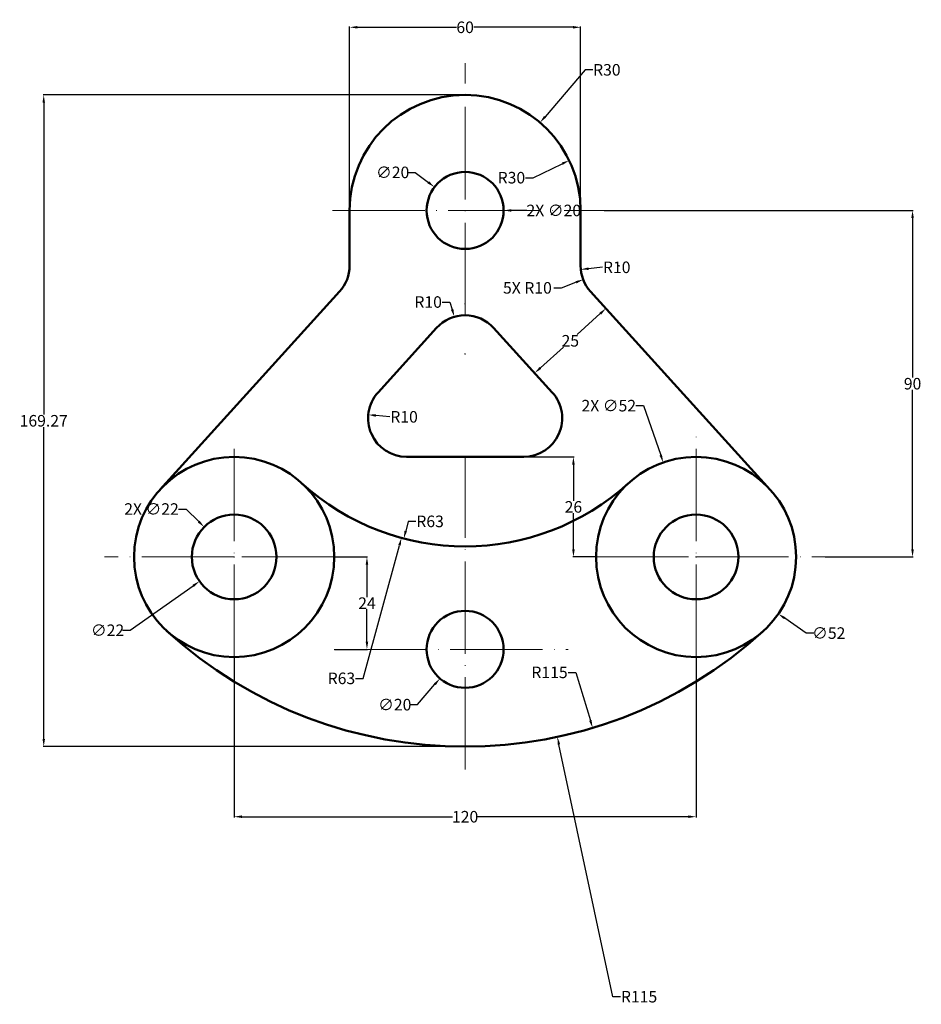
# Model space of a CAD drawing. Units: inches. Extents: x 239 to 473, y 124 to 379.
import ezdxf

# ---------------------------------------------------------------- set-up
doc = ezdxf.new("R2010")
doc.units = ezdxf.units.IN
doc.header["$MEASUREMENT"] = 0
doc.linetypes.add('ACAD_ISO04W100', pattern=[30, 24, -3, 0, -3])
for name, color, linetype, lineweight in [('M-CNTR', 4, 'ACAD_ISO04W100', 18), ('M-DIMS', 2, 'Continuous', 25), ('M-OUTL', 7, 'Continuous', 50)]:
    doc.layers.add(name, color=color, linetype=linetype, lineweight=lineweight)
doc.styles.get("Standard").update_dxf_attribs({"font": 'arial.ttf'})
doc.dimstyles.get("Standard").update_dxf_attribs({"dimtxt": 3, "dimasz": 2, "dimexe": 0.18, "dimexo": 0.0625, "dimgap": 0.09, "dimtad": 0, "dimtih": 1, "dimtoh": 1, "dimdec": 0, "dimzin": 0, "dimdsep": 46, "dimtxsty": 'Standard', "dimcen": 0.09, "dimadec": 0, "dimazin": 0, "dimtfac": 1, "dimtdec": 0, "dimtofl": 0, "dimtmove": 0, "dimatfit": 3, "dimfxl": 1, "dimtolj": 1, "dimtzin": 0, "dimarcsym": 0})

# ---------------------------------------------------------------- blocks, each defined once
blk = doc.blocks.new('*D1')
at = {"layer": 'Defpoints', "color": 0, "transparency": 16777216}
for p in [(381.57, 342.88), (354.54, 329.88)]:
    blk.add_point(p, dxfattribs=at)
at = {"layer": 'M-DIMS', "color": 0, "lineweight": -2, "transparency": 16777216}
for p, q in [((372.23, 338.39), (379.77, 342.02)), ((370.23, 338.39), (372.23, 338.39))]:
    blk.add_line(p, q, dxfattribs=at)
at = {"layer": 'M-DIMS', "color": 0, "transparency": 16777216}
blk.add_solid([(379.63, 342.32), (379.91, 341.72), (381.57, 342.88)], dxfattribs=at)
at = {"layer": 'M-DIMS', "color": 0, "transparency": 16777216, "insert": (366.56, 338.39), "char_height": 3, "attachment_point": 5}
blk.add_mtext('\\A1;R30', dxfattribs=at)
blk = doc.blocks.new('*D2')
at = {"layer": 'Defpoints', "color": 0, "transparency": 16777216}
for p in [(346.59, 335.95), (362.49, 323.82)]:
    blk.add_point(p, dxfattribs=at)
at = {"layer": 'M-DIMS', "color": 0, "lineweight": -2, "transparency": 16777216}
for p, q in [((339.58, 339.77), (341.58, 339.77)), ((341.58, 339.77), (345, 337.16)), ((354.54, 329.79), (354.54, 329.97)), ((354.45, 329.88), (354.63, 329.88))]:
    blk.add_line(p, q, dxfattribs=at)
at = {"layer": 'M-DIMS', "color": 0, "transparency": 16777216}
blk.add_solid([(345.2, 337.43), (344.79, 336.9), (346.59, 335.95)], dxfattribs=at)
at = {"layer": 'M-DIMS', "color": 0, "transparency": 16777216, "insert": (335.72, 339.77), "char_height": 3, "attachment_point": 5}
blk.add_mtext('\\A1;∅20', dxfattribs=at)
blk = doc.blocks.new('*D3')
at = {"layer": 'Defpoints', "color": 0, "transparency": 16777216}
for p in [(390.61, 329.88), (448.02, 239.88), (470.77, 239.88)]:
    blk.add_point(p, dxfattribs=at)
at = {"layer": 'M-DIMS', "color": 0, "lineweight": -2, "transparency": 16777216}
for p, q in [((390.67, 329.88), (470.95, 329.88)), ((470.77, 327.88), (470.77, 286.5)), ((470.77, 241.88), (470.77, 283.26)), ((448.08, 239.88), (470.95, 239.88))]:
    blk.add_line(p, q, dxfattribs=at)
at = {"layer": 'M-DIMS', "color": 0, "transparency": 16777216}
for points in [[(470.43, 327.88), (471.1, 327.88), (470.77, 329.88)], [(470.43, 241.88), (471.1, 241.88), (470.77, 239.88)]]:
    blk.add_solid(points, dxfattribs=at)
at = {"layer": 'M-DIMS', "color": 0, "transparency": 16777216, "insert": (470.77, 284.88), "char_height": 3, "attachment_point": 5}
blk.add_mtext('\\A1;90', dxfattribs=at)
blk = doc.blocks.new('*D4')
at = {"layer": 'Defpoints', "color": 0, "transparency": 16777216}
for p in [(354.54, 305.62), (338.61, 244.66)]:
    blk.add_point(p, dxfattribs=at)
at = {"layer": 'M-DIMS', "color": 0, "lineweight": -2, "transparency": 16777216}
for p, q in [((339.77, 249.12), (339.11, 246.6)), ((341.77, 249.12), (339.77, 249.12))]:
    blk.add_line(p, q, dxfattribs=at)
at = {"layer": 'M-DIMS', "color": 0, "transparency": 16777216}
blk.add_solid([(338.79, 246.68), (339.43, 246.52), (338.61, 244.66)], dxfattribs=at)
at = {"layer": 'M-DIMS', "color": 0, "transparency": 16777216, "insert": (345.44, 249.12), "char_height": 3, "attachment_point": 5}
blk.add_mtext('\\A1;R63', dxfattribs=at)
blk = doc.blocks.new('*D5')
at = {"layer": 'Defpoints', "color": 0, "transparency": 16777216}
for p in [(303.53, 246.22), (285.54, 233.55)]:
    blk.add_point(p, dxfattribs=at)
at = {"layer": 'M-DIMS', "color": 0, "lineweight": -2, "transparency": 16777216}
for p, q in [((294.45, 239.88), (294.63, 239.88)), ((294.54, 239.79), (294.54, 239.97)), ((267.52, 220.84), (283.91, 232.39)), ((265.52, 220.84), (267.52, 220.84))]:
    blk.add_line(p, q, dxfattribs=at)
at = {"layer": 'M-DIMS', "color": 0, "transparency": 16777216}
blk.add_solid([(283.72, 232.67), (284.1, 232.12), (285.54, 233.55)], dxfattribs=at)
at = {"layer": 'M-DIMS', "color": 0, "transparency": 16777216, "insert": (261.66, 220.84), "char_height": 3, "attachment_point": 5}
blk.add_mtext('\\A1;∅22', dxfattribs=at)
blk = doc.blocks.new('*D6')
at = {"layer": 'Defpoints', "color": 0, "transparency": 16777216}
for p in [(393.15, 254.67), (435.92, 225.1)]:
    blk.add_point(p, dxfattribs=at)
at = {"layer": 'M-DIMS', "color": 0, "lineweight": -2, "transparency": 16777216}
for p, q in [((414.45, 239.88), (414.63, 239.88)), ((414.54, 239.79), (414.54, 239.97)), ((443.13, 220.11), (437.57, 223.96)), ((445.13, 220.11), (443.13, 220.11))]:
    blk.add_line(p, q, dxfattribs=at)
at = {"layer": 'M-DIMS', "color": 0, "transparency": 16777216}
blk.add_solid([(437.76, 224.23), (437.38, 223.68), (435.92, 225.1)], dxfattribs=at)
at = {"layer": 'M-DIMS', "color": 0, "transparency": 16777216, "insert": (448.99, 220.11), "char_height": 3, "attachment_point": 5}
blk.add_mtext('\\A1;∅52', dxfattribs=at)
blk = doc.blocks.new('*D7')
at = {"layer": 'Defpoints', "color": 0, "transparency": 16777216}
for p in [(354.54, 305.62), (387.65, 195.49)]:
    blk.add_point(p, dxfattribs=at)
at = {"layer": 'M-DIMS', "color": 0, "lineweight": -2, "transparency": 16777216}
for p, q in [((381.31, 209.9), (383.31, 209.9)), ((383.31, 209.9), (387.07, 197.4))]:
    blk.add_line(p, q, dxfattribs=at)
at = {"layer": 'M-DIMS', "color": 0, "transparency": 16777216}
blk.add_solid([(387.39, 197.5), (386.75, 197.31), (387.65, 195.49)], dxfattribs=at)
at = {"layer": 'M-DIMS', "color": 0, "transparency": 16777216, "insert": (376.46, 209.9), "char_height": 3, "attachment_point": 5}
blk.add_mtext('\\A1;R115', dxfattribs=at)
blk = doc.blocks.new('*D8')
at = {"layer": 'Defpoints', "color": 0, "transparency": 16777216}
for p in [(361.07, 223.45), (348, 208.32)]:
    blk.add_point(p, dxfattribs=at)
at = {"layer": 'M-DIMS', "color": 0, "lineweight": -2, "transparency": 16777216}
for p, q in [((354.45, 215.88), (354.63, 215.88)), ((354.54, 215.79), (354.54, 215.97)), ((342.13, 201.52), (346.69, 206.8)), ((340.13, 201.52), (342.13, 201.52))]:
    blk.add_line(p, q, dxfattribs=at)
at = {"layer": 'M-DIMS', "color": 0, "transparency": 16777216}
blk.add_solid([(346.44, 207.02), (346.94, 206.58), (348, 208.32)], dxfattribs=at)
at = {"layer": 'M-DIMS', "color": 0, "transparency": 16777216, "insert": (336.26, 201.52), "char_height": 3, "attachment_point": 5}
blk.add_mtext('\\A1;∅20', dxfattribs=at)
blk = doc.blocks.new('*D9')
at = {"layer": 'Defpoints', "color": 0, "transparency": 16777216}
for p in [(320.54, 239.88), (320.54, 215.88), (329.04, 215.88)]:
    blk.add_point(p, dxfattribs=at)
at = {"layer": 'M-DIMS', "color": 0, "lineweight": -2, "transparency": 16777216}
for p, q in [((320.6, 239.88), (329.22, 239.88)), ((329.04, 237.88), (329.04, 229.48)), ((329.04, 217.88), (329.04, 226.29)), ((320.6, 215.88), (329.22, 215.88))]:
    blk.add_line(p, q, dxfattribs=at)
at = {"layer": 'M-DIMS', "color": 0, "transparency": 16777216}
for points in [[(328.71, 237.88), (329.37, 237.88), (329.04, 239.88)], [(328.71, 217.88), (329.37, 217.88), (329.04, 215.88)]]:
    blk.add_solid(points, dxfattribs=at)
at = {"layer": 'M-DIMS', "color": 0, "transparency": 16777216, "insert": (329.04, 227.88), "char_height": 3, "attachment_point": 5}
blk.add_mtext('\\A1;24', dxfattribs=at)
blk = doc.blocks.new('*D10')
at = {"layer": 'Defpoints', "color": 0, "transparency": 16777216}
for p in [(384.58, 314.57), (394.54, 315.54)]:
    blk.add_point(p, dxfattribs=at)
at = {"layer": 'M-DIMS', "color": 0, "lineweight": -2, "transparency": 16777216}
blk.add_line((390.25, 315.12), (386.57, 314.76), dxfattribs=at)
at = {"layer": 'M-DIMS', "color": 0, "transparency": 16777216}
blk.add_solid([(386.54, 315.09), (386.61, 314.43), (384.58, 314.57)], dxfattribs=at)
at = {"layer": 'M-DIMS', "color": 0, "transparency": 16777216, "insert": (393.92, 315.12), "char_height": 3, "attachment_point": 5}
blk.add_mtext('\\A1;R10', dxfattribs=at)
blk = doc.blocks.new('*D11')
at = {"layer": 'Defpoints', "color": 0, "transparency": 16777216}
for p in [(384.54, 377.46), (324.54, 329.88), (384.54, 329.88)]:
    blk.add_point(p, dxfattribs=at)
at = {"layer": 'M-DIMS', "color": 0, "lineweight": -2, "transparency": 16777216}
for p, q in [((324.54, 329.95), (324.54, 377.64)), ((326.54, 377.46), (352.29, 377.46)), ((382.54, 377.46), (356.78, 377.46)), ((384.54, 329.95), (384.54, 377.64))]:
    blk.add_line(p, q, dxfattribs=at)
at = {"layer": 'M-DIMS', "color": 0, "transparency": 16777216}
for points in [[(326.54, 377.79), (326.54, 377.13), (324.54, 377.46)], [(382.54, 377.79), (382.54, 377.13), (384.54, 377.46)]]:
    blk.add_solid(points, dxfattribs=at)
at = {"layer": 'M-DIMS', "color": 0, "transparency": 16777216, "insert": (354.54, 377.46), "char_height": 3, "attachment_point": 5}
blk.add_mtext('\\A1;60', dxfattribs=at)
blk = doc.blocks.new('*D12')
at = {"layer": 'Defpoints', "color": 0, "transparency": 16777216}
for p in [(294.54, 213.88), (414.54, 213.88), (414.54, 172.41)]:
    blk.add_point(p, dxfattribs=at)
at = {"layer": 'M-DIMS', "color": 0, "lineweight": -2, "transparency": 16777216}
for p, q in [((294.54, 213.82), (294.54, 172.23)), ((414.54, 213.82), (414.54, 172.23)), ((296.54, 172.41), (351.28, 172.41)), ((412.54, 172.41), (357.79, 172.41))]:
    blk.add_line(p, q, dxfattribs=at)
at = {"layer": 'M-DIMS', "color": 0, "transparency": 16777216}
for points in [[(296.54, 172.75), (296.54, 172.08), (294.54, 172.41)], [(412.54, 172.75), (412.54, 172.08), (414.54, 172.41)]]:
    blk.add_solid(points, dxfattribs=at)
at = {"layer": 'M-DIMS', "color": 0, "transparency": 16777216, "insert": (354.54, 172.41), "char_height": 3, "attachment_point": 5}
blk.add_mtext('\\A1;120', dxfattribs=at)
blk = doc.blocks.new('*D13')
at = {"layer": 'Defpoints', "color": 0, "transparency": 16777216}
for p in [(391.12, 304.42), (369.22, 291.36), (372.6, 287.63)]:
    blk.add_point(p, dxfattribs=at)
at = {"layer": 'M-DIMS', "color": 0, "lineweight": -2, "transparency": 16777216}
for p, q in [((391.07, 304.47), (391, 304.56)), ((389.63, 303.08), (383.64, 297.65)), ((374.08, 288.97), (380.07, 294.41)), ((369.26, 291.31), (372.72, 287.5))]:
    blk.add_line(p, q, dxfattribs=at)
at = {"layer": 'M-DIMS', "color": 0, "transparency": 16777216}
for points in [[(389.41, 303.33), (389.86, 302.83), (391.12, 304.42)], [(373.85, 289.22), (374.3, 288.73), (372.6, 287.63)]]:
    blk.add_solid(points, dxfattribs=at)
at = {"layer": 'M-DIMS', "color": 0, "transparency": 16777216, "insert": (381.86, 296.03), "char_height": 3, "attachment_point": 5}
blk.add_mtext('\\A1;25', dxfattribs=at)
blk = doc.blocks.new('*D14')
at = {"layer": 'Defpoints', "color": 0, "transparency": 16777216}
for p in [(329.37, 276.81), (339.32, 275.88)]:
    blk.add_point(p, dxfattribs=at)
at = {"layer": 'M-DIMS', "color": 0, "lineweight": -2, "transparency": 16777216}
blk.add_line((335.01, 276.28), (331.36, 276.62), dxfattribs=at)
at = {"layer": 'M-DIMS', "color": 0, "transparency": 16777216}
blk.add_solid([(331.39, 276.96), (331.33, 276.29), (329.37, 276.81)], dxfattribs=at)
at = {"layer": 'M-DIMS', "color": 0, "transparency": 16777216, "insert": (338.68, 276.28), "char_height": 3, "attachment_point": 5}
blk.add_mtext('\\A1;R10', dxfattribs=at)
blk = doc.blocks.new('*D15')
at = {"layer": 'Defpoints', "color": 0, "transparency": 16777216}
for p in [(351.73, 302.26), (354.54, 292.66)]:
    blk.add_point(p, dxfattribs=at)
at = {"layer": 'M-DIMS', "color": 0, "lineweight": -2, "transparency": 16777216}
for p, q in [((348.61, 306.1), (350.61, 306.1)), ((350.61, 306.1), (351.17, 304.18)), ((354.45, 292.66), (354.63, 292.66)), ((354.54, 292.57), (354.54, 292.75))]:
    blk.add_line(p, q, dxfattribs=at)
at = {"layer": 'M-DIMS', "color": 0, "transparency": 16777216}
blk.add_solid([(351.49, 304.27), (350.85, 304.09), (351.73, 302.26)], dxfattribs=at)
at = {"layer": 'M-DIMS', "color": 0, "transparency": 16777216, "insert": (344.94, 306.1), "char_height": 3, "attachment_point": 5}
blk.add_mtext('\\A1;R10', dxfattribs=at)
blk = doc.blocks.new('*D16')
at = {"layer": 'Defpoints', "color": 0, "transparency": 16777216}
for p in [(369.75, 265.88), (382.67, 265.88), (388.54, 239.88)]:
    blk.add_point(p, dxfattribs=at)
at = {"layer": 'M-DIMS', "color": 0, "lineweight": -2, "transparency": 16777216}
for p, q in [((369.81, 265.88), (382.85, 265.88)), ((382.67, 263.88), (382.67, 254.5)), ((382.67, 241.88), (382.67, 251.26)), ((388.47, 239.88), (382.49, 239.88))]:
    blk.add_line(p, q, dxfattribs=at)
at = {"layer": 'M-DIMS', "color": 0, "transparency": 16777216}
for points in [[(382.34, 263.88), (383.01, 263.88), (382.67, 265.88)], [(382.34, 241.88), (383.01, 241.88), (382.67, 239.88)]]:
    blk.add_solid(points, dxfattribs=at)
at = {"layer": 'M-DIMS', "color": 0, "transparency": 16777216, "insert": (382.67, 252.88), "char_height": 3, "attachment_point": 5}
blk.add_mtext('\\A1;26', dxfattribs=at)
blk = doc.blocks.new('MOUNTING-LOBE-52-BORE-22')
for radius in [26, 11]:
    blk.add_circle((26, 26), radius)
blk = doc.blocks.new('HOLE-D20')
blk.add_circle((10, 10), 10)
blk = doc.blocks.new('*D19')
at = {"layer": 'Defpoints', "color": 0, "transparency": 16777216}
for p in [(245.08, 359.88), (354.54, 359.88), (354.54, 190.62)]:
    blk.add_point(p, dxfattribs=at)
at = {"layer": 'M-DIMS', "color": 0, "lineweight": -2, "transparency": 16777216}
for p, q in [((354.47, 359.88), (244.9, 359.88)), ((245.08, 357.88), (245.08, 276.87)), ((245.08, 192.62), (245.08, 273.63)), ((354.47, 190.62), (244.9, 190.62))]:
    blk.add_line(p, q, dxfattribs=at)
at = {"layer": 'M-DIMS', "color": 0, "transparency": 16777216}
for points in [[(244.75, 357.88), (245.41, 357.88), (245.08, 359.88)], [(244.75, 192.62), (245.41, 192.62), (245.08, 190.62)]]:
    blk.add_solid(points, dxfattribs=at)
at = {"layer": 'M-DIMS', "color": 0, "transparency": 16777216, "insert": (245.08, 275.25), "char_height": 3, "attachment_point": 5}
blk.add_mtext('\\A1;169.27', dxfattribs=at)
blk = doc.blocks.new('*D20')
at = {"layer": 'Defpoints', "color": 0, "transparency": 16777216}
for p in [(406, 264.44), (423.07, 215.32)]:
    blk.add_point(p, dxfattribs=at)
at = {"layer": 'M-DIMS', "color": 0, "lineweight": -2, "transparency": 16777216}
for p, q in [((398.88, 279.18), (400.88, 279.18)), ((400.88, 279.18), (405.34, 266.33)), ((414.45, 239.88), (414.63, 239.88)), ((414.54, 239.79), (414.54, 239.97))]:
    blk.add_line(p, q, dxfattribs=at)
at = {"layer": 'M-DIMS', "color": 0, "transparency": 16777216}
blk.add_solid([(405.66, 266.44), (405.03, 266.22), (406, 264.44)], dxfattribs=at)
at = {"layer": 'M-DIMS', "color": 0, "transparency": 16777216, "insert": (391.85, 279.18), "char_height": 3, "attachment_point": 5}
blk.add_mtext('\\A1;2X ∅52', dxfattribs=at)
blk = doc.blocks.new('*D21')
at = {"layer": 'Defpoints', "color": 0, "transparency": 16777216}
for p in [(286.76, 247.66), (302.31, 232.1)]:
    blk.add_point(p, dxfattribs=at)
at = {"layer": 'M-DIMS', "color": 0, "lineweight": -2, "transparency": 16777216}
for p, q in [((280.09, 252.33), (282.09, 252.33)), ((282.09, 252.33), (285.34, 249.08)), ((294.45, 239.88), (294.63, 239.88)), ((294.54, 239.79), (294.54, 239.97))]:
    blk.add_line(p, q, dxfattribs=at)
at = {"layer": 'M-DIMS', "color": 0, "transparency": 16777216}
blk.add_solid([(285.58, 249.31), (285.11, 248.84), (286.76, 247.66)], dxfattribs=at)
at = {"layer": 'M-DIMS', "color": 0, "transparency": 16777216, "insert": (273.07, 252.33), "char_height": 3, "attachment_point": 5}
blk.add_mtext('\\A1;2X ∅22', dxfattribs=at)
blk = doc.blocks.new('*D22')
at = {"layer": 'Defpoints', "color": 0, "transparency": 16777216}
for p in [(344.54, 329.88), (364.54, 329.88)]:
    blk.add_point(p, dxfattribs=at)
at = {"layer": 'M-DIMS', "color": 0, "lineweight": -2, "transparency": 16777216}
for p, q in [((354.54, 329.79), (354.54, 329.97)), ((354.45, 329.88), (354.63, 329.88)), ((370.54, 329.88), (366.54, 329.88))]:
    blk.add_line(p, q, dxfattribs=at)
at = {"layer": 'M-DIMS', "color": 0, "transparency": 16777216}
blk.add_solid([(366.54, 330.22), (366.54, 329.55), (364.54, 329.88)], dxfattribs=at)
at = {"layer": 'M-DIMS', "color": 0, "transparency": 16777216, "insert": (377.57, 329.88), "char_height": 3, "attachment_point": 5}
blk.add_mtext('\\A1;2X ∅20', dxfattribs=at)
blk = doc.blocks.new('*D23')
at = {"layer": 'Defpoints', "color": 0, "transparency": 16777216}
for p in [(354.54, 305.62), (378.5, 193.14)]:
    blk.add_point(p, dxfattribs=at)
at = {"layer": 'M-DIMS', "color": 0, "lineweight": -2, "transparency": 16777216}
for p, q in [((354.45, 305.62), (354.63, 305.62)), ((354.54, 305.53), (354.54, 305.71)), ((392.88, 125.66), (378.92, 191.19)), ((394.88, 125.66), (392.88, 125.66))]:
    blk.add_line(p, q, dxfattribs=at)
at = {"layer": 'M-DIMS', "color": 0, "transparency": 16777216}
blk.add_solid([(379.24, 191.26), (378.59, 191.12), (378.5, 193.14)], dxfattribs=at)
at = {"layer": 'M-DIMS', "color": 0, "transparency": 16777216, "insert": (399.73, 125.66), "char_height": 3, "attachment_point": 5}
blk.add_mtext('\\A1;R115', dxfattribs=at)
blk = doc.blocks.new('*D24')
at = {"layer": 'Defpoints', "color": 0, "transparency": 16777216}
for p in [(354.54, 305.62), (338, 244.83)]:
    blk.add_point(p, dxfattribs=at)
at = {"layer": 'M-DIMS', "color": 0, "lineweight": -2, "transparency": 16777216}
for p, q in [((354.45, 305.62), (354.63, 305.62)), ((354.54, 305.53), (354.54, 305.71)), ((328.08, 208.35), (337.48, 242.9)), ((326.08, 208.35), (328.08, 208.35))]:
    blk.add_line(p, q, dxfattribs=at)
at = {"layer": 'M-DIMS', "color": 0, "transparency": 16777216}
blk.add_solid([(337.16, 242.98), (337.8, 242.81), (338, 244.83)], dxfattribs=at)
at = {"layer": 'M-DIMS', "color": 0, "transparency": 16777216, "insert": (322.41, 208.35), "char_height": 3, "attachment_point": 5}
blk.add_mtext('\\A1;R63', dxfattribs=at)
blk = doc.blocks.new('*D25')
at = {"layer": 'Defpoints', "color": 0, "transparency": 16777216}
for p in [(374, 352.71), (354.54, 329.88)]:
    blk.add_point(p, dxfattribs=at)
at = {"layer": 'M-DIMS', "color": 0, "lineweight": -2, "transparency": 16777216}
for p, q in [((385.68, 366.41), (375.3, 354.24)), ((387.68, 366.41), (385.68, 366.41)), ((354.54, 329.79), (354.54, 329.97)), ((354.45, 329.88), (354.63, 329.88))]:
    blk.add_line(p, q, dxfattribs=at)
at = {"layer": 'M-DIMS', "color": 0, "transparency": 16777216}
blk.add_solid([(375.04, 354.45), (375.55, 354.02), (374, 352.71)], dxfattribs=at)
at = {"layer": 'M-DIMS', "color": 0, "transparency": 16777216, "insert": (391.35, 366.41), "char_height": 3, "attachment_point": 5}
blk.add_mtext('\\A1;R30', dxfattribs=at)
blk = doc.blocks.new('*D26')
at = {"layer": 'Defpoints', "color": 0, "transparency": 16777216}
for p in [(394.54, 315.54), (385.21, 311.94)]:
    blk.add_point(p, dxfattribs=at)
at = {"layer": 'M-DIMS', "color": 0, "lineweight": -2, "transparency": 16777216}
for p, q in [((394.45, 315.54), (394.63, 315.54)), ((394.54, 315.45), (394.54, 315.63)), ((377.61, 309.78), (379.61, 309.78)), ((379.61, 309.78), (383.34, 311.22))]:
    blk.add_line(p, q, dxfattribs=at)
at = {"layer": 'M-DIMS', "color": 0, "transparency": 16777216}
blk.add_solid([(383.22, 311.53), (383.46, 310.91), (385.21, 311.94)], dxfattribs=at)
at = {"layer": 'M-DIMS', "color": 0, "transparency": 16777216, "insert": (370.72, 309.78), "char_height": 3, "attachment_point": 5}
blk.add_mtext('\\A1;5X R10', dxfattribs=at)

msp = doc.modelspace()

# ---------------------------------------------------------------- linework, layer by layer
at = {"layer": 'M-CNTR'}
for p, q in [((354.536, 302.663), (354.536, 368.175)), ((320.048, 329.883), (390.607, 329.883)), ((414.536, 213.883), (414.536, 272.304)), ((294.536, 213.883), (294.536, 270.408)), ((354.536, 184.639), (354.536, 265.883)), ((294.536, 239.883), (260.829, 239.883)), ((320.536, 239.883), (294.536, 239.883)), ((320.536, 215.883), (381.327, 215.883))]:
    msp.add_line(p, q, dxfattribs=at)
msp.add_lwpolyline([(388.536, 239.883), (414.536, 239.883), (448.02, 239.883)], dxfattribs=at)
at = {"layer": 'M-OUTL'}
for p, q in [((324.536, 329.883), (324.536, 315.54)), ((384.536, 329.883), (384.536, 315.54)), ((275.274, 257.347), (321.944, 308.823)), ((387.127, 308.823), (433.798, 257.347)), ((331.914, 282.6), (347.127, 299.379)), ((377.157, 282.6), (361.944, 299.379)), ((354.536, 265.883), (339.323, 265.883)), ((354.536, 265.883), (369.749, 265.883))]:
    msp.add_line(p, q, dxfattribs=at)
for centre, radius, start, end in [((354.536, 329.883), 30, 0, 180), ((314.536, 315.54), 10, 317.80352, 0), ((394.536, 315.54), 10, 180, 222.19648), ((354.536, 292.663), 10, 42.19648, 137.80352), ((339.323, 275.883), 10, 137.80352, 270), ((369.749, 275.883), 10, 270, 42.19648), ((354.536, 305.617), 63, 227.61126, 312.38874), ((354.536, 305.617), 115, 227.61126, 312.38874)]:
    msp.add_arc(centre, radius, start, end, dxfattribs=at)

# ---------------------------------------------------------------- block references
for name, p in [('HOLE-D20', (344.536, 319.883)), ('MOUNTING-LOBE-52-BORE-22', (268.536, 213.883)), ('MOUNTING-LOBE-52-BORE-22', (388.536, 213.883)), ('HOLE-D20', (344.536, 205.883))]:
    msp.add_blockref(name, p, dxfattribs=at)

# ---------------------------------------------------------------- dimensions: what is measured, and where the dimension line sits
at = {"layer": 'M-DIMS'}
for base, p1, p2, picture, middle in [((384.536, 377.461), (324.536, 329.883), (384.536, 329.883), '*D11', (354.536, 377.461)), ((414.536, 172.415), (294.536, 213.883), (414.536, 213.883), '*D12', (354.536, 172.415))]:
    dim = msp.add_linear_dim(base=base, p1=p1, p2=p2, dimstyle='Standard', override={"dimclrd": 0, "dimclre": 0, "dimclrt": 0}, dxfattribs=at)
    dim.commit()
    dim.dimension.update_dxf_attribs({"geometry": picture, "text_midpoint": middle})
for center, mpoint, override, picture, middle in [((354.536, 329.883), (373.998, 352.713), {"dimdec": 0, "dimlfac": 1, "dimrnd": 0, "dimzin": 0, "dimdsep": 46, "dimlunit": 2}, '*D25', (391.345, 366.411)), ((354.536, 329.883), (381.572, 342.884), {"dimclrd": 0, "dimclre": 0, "dimclrt": 0}, '*D1', (366.562, 338.392)), ((394.536, 315.54), (384.583, 314.565), {"dimclrd": 0, "dimclre": 0, "dimclrt": 0}, '*D10', (390.246, 315.12)), ((354.536, 305.617), (338.002, 244.826), {"dimdec": 0, "dimlfac": 1, "dimrnd": 0, "dimzin": 0, "dimdsep": 46, "dimlunit": 2}, '*D24', (322.407, 208.351)), ((354.536, 305.617), (338.606, 244.665), {"dimclrd": 0, "dimclre": 0, "dimclrt": 0}, '*D4', (345.443, 249.115)), ((354.536, 305.617), (378.5, 193.142), {"dimdec": 0, "dimlfac": 1, "dimrnd": 0, "dimzin": 0, "dimdsep": 46, "dimlunit": 2}, '*D23', (399.729, 125.657)), ((354.536, 305.617), (387.646, 195.487), {"dimclrd": 0, "dimclre": 0, "dimclrt": 0}, '*D7', (376.463, 209.897)), ((339.323, 275.883), (329.366, 276.81), {"dimclrd": 0, "dimclre": 0, "dimclrt": 0}, '*D14', (335.009, 276.285))]:
    dim = msp.add_radius_dim(center=center, mpoint=mpoint, dimstyle='Standard', override=override, dxfattribs=at)
    dim.commit()
    dim.dimension.update_dxf_attribs({"geometry": picture, "text_midpoint": middle, "dimtype": 164})
for base, p1, p2, angle, override, picture, middle in [((245.079, 359.883), (354.536, 190.617), (354.536, 359.883), 90, {"dimdec": 2, "dimlfac": 1, "dimrnd": 0, "dimzin": 0, "dimdsep": 46, "dimlunit": 2}, '*D19', (245.079, 275.25)), ((470.768, 239.883), (390.607, 329.883), (448.02, 239.883), 90, {"dimclrd": 0, "dimclre": 0, "dimclrt": 0}, '*D3', (470.768, 284.883)), ((372.595, 287.632), (391.116, 304.424), (369.217, 291.358), 42.19648, {"dimclrd": 0, "dimclre": 0, "dimclrt": 0}, '*D13', (381.856, 296.028)), ((382.674, 265.883), (388.536, 239.883), (369.749, 265.883), 90, {"dimclrd": 0, "dimclre": 0, "dimclrt": 0}, '*D16', (382.674, 252.883)), ((329.041, 215.883), (320.536, 239.883), (320.536, 215.883), 90, {"dimclrd": 0, "dimclre": 0, "dimclrt": 0}, '*D9', (329.041, 227.883))]:
    dim = msp.add_linear_dim(base=base, p1=p1, p2=p2, angle=angle, dimstyle='Standard', override=override, dxfattribs=at)
    dim.commit()
    dim.dimension.update_dxf_attribs({"geometry": picture, "text_midpoint": middle})
for p1, p2, picture, middle in [((362.486, 323.818), (346.585, 335.948), '*D2', (335.716, 339.766)), ((393.151, 254.671), (435.921, 225.095), '*D6', (448.986, 220.109)), ((303.527, 246.22), (285.544, 233.546), '*D5', (261.66, 220.84)), ((361.074, 223.45), (347.998, 208.316), '*D8', (336.26, 201.519))]:
    dim = msp.add_diameter_dim_2p(p1=p1, p2=p2, dimstyle='Standard', override={"dimclrd": 0, "dimclre": 0, "dimclrt": 0}, dxfattribs=at)
    dim.commit()
    dim.dimension.update_dxf_attribs({"geometry": picture, "text_midpoint": middle, "dimtype": 163})
for p1, p2, picture, middle in [((344.536, 329.883), (364.536, 329.883), '*D22', (370.536, 329.883)), ((423.072, 215.324), (405.999, 264.442), '*D20', (391.853, 279.177)), ((302.313, 232.104), (286.758, 247.662), '*D21', (273.067, 252.329))]:
    dim = msp.add_diameter_dim_2p(p1=p1, p2=p2, text='2X <>', dimstyle='Standard', override={"dimdec": 0, "dimlfac": 1, "dimrnd": 0, "dimzin": 0, "dimdsep": 46, "dimlunit": 2}, dxfattribs=at)
    dim.commit()
    dim.dimension.update_dxf_attribs({"geometry": picture, "text_midpoint": middle, "dimtype": 163})
dim = msp.add_radius_dim(center=(394.536, 315.54), mpoint=(385.206, 311.94), text='5X <>', dimstyle='Standard', override={"dimdec": 0, "dimlfac": 1, "dimrnd": 0, "dimzin": 0, "dimdsep": 46, "dimlunit": 2}, dxfattribs=at)
dim.commit()
dim.dimension.update_dxf_attribs({"geometry": '*D26', "text_midpoint": (370.716, 309.78), "dimtype": 164})
dim = msp.add_radius_dim(center=(354.536, 292.663), mpoint=(351.732, 302.262), dimstyle='Standard', override={"dimclrd": 0, "dimclre": 0, "dimclrt": 0}, dxfattribs=at)
dim.commit()
dim.dimension.update_dxf_attribs({"geometry": '*D15', "text_midpoint": (344.942, 306.101)})

doc.saveas('drawing.dxf')
